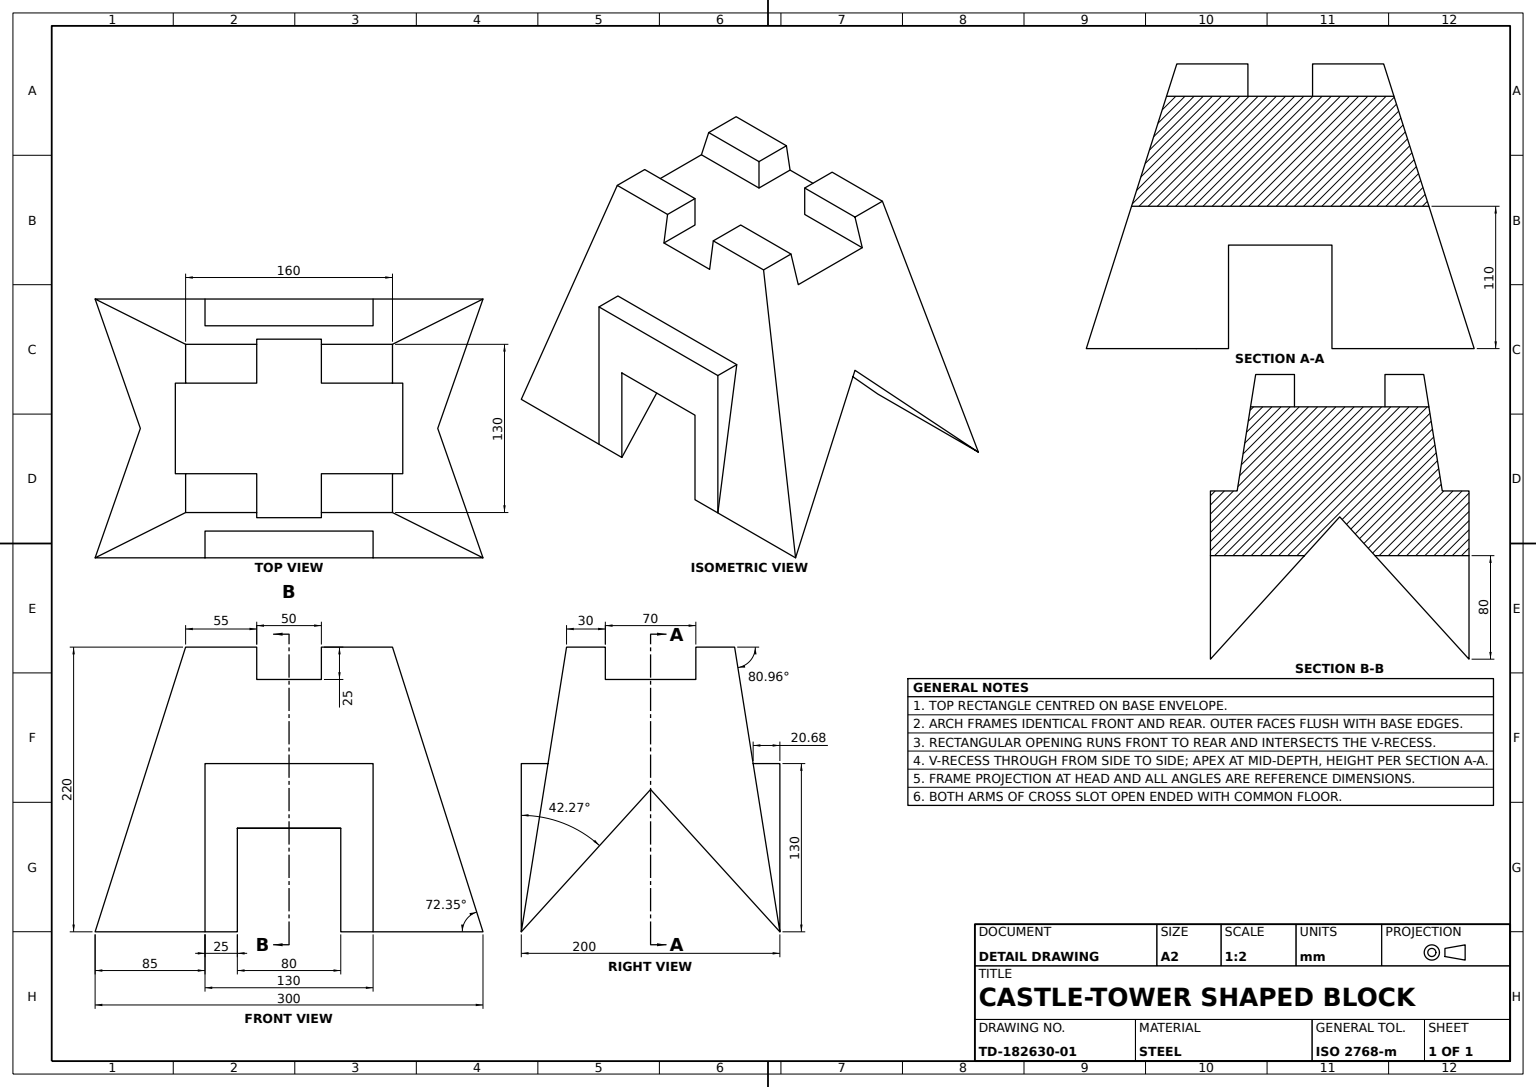
from build123d import *

# Parameters (mm, degrees)
INCLINED_BASE_BLOCK_DEPTH           = 100
FRONT_NOTCH_CUT_DEPTH               = 285.429253067
FRONT_NOTCH_CUT_DEPTH_BACK          = 285.429253067
FRONT_NOTCH_SKETCH_OUTSIDE_W        = 286.474
FRONT_NOTCH_SKETCH_OUTSIDE_H        = 306.474
TOP_RECESS_CUT_DEPTH                = 285.429253067
TOP_RECESS_CUT_DEPTH_BACK           = 285.429253067
FRONT_FRAME_BOSS_DEPTH              = 65
TOP_CROSS_SLOT_CUT_80X80_DEPTH      = 334.016516107
TOP_CROSS_SLOT_CUT_80X80_DEPTH_BACK = 334.016516107
TOP_CROSS_SLOT_SKETCH_W             = 80
TOP_CROSS_SLOT_SKETCH_H             = 80


with BuildPart() as part:
    # Base Profile Sketch → Inclined Base Block (new, symmetric)
    with BuildSketch(Plane(origin=(0, 0, 0), x_dir=(0, 0, -1), z_dir=(1, 0, 0))):
        Polygon((-150, 0), (-80, 220), (-25, 220), (-25, 195), (25, 195), (25, 220), (80, 220), (150, 0), align=None)
    extrude(amount=INCLINED_BASE_BLOCK_DEPTH, both=True)

    # Front Notch Sketch outside → Front Notch Cut (cut, two sides: drawn at the far end of the back side and taken through both)
    with BuildSketch(Plane.XY.offset(-FRONT_NOTCH_CUT_DEPTH_BACK)):
        with Locations((0, 110)):
            Rectangle(FRONT_NOTCH_SKETCH_OUTSIDE_W, FRONT_NOTCH_SKETCH_OUTSIDE_H)
        Polygon((-100, 0), (-65, 220), (-35, 220), (-35, 195), (35, 195), (35, 220), (65, 220), (100, 0), align=None, mode=Mode.SUBTRACT)
    extrude(amount=FRONT_NOTCH_CUT_DEPTH + FRONT_NOTCH_CUT_DEPTH_BACK, mode=Mode.SUBTRACT)

    # Top Recess Sketch → Top Recess Cut (cut, two sides: drawn at the far end of the back side and taken through both)
    with BuildSketch(Plane.XY.offset(-TOP_RECESS_CUT_DEPTH_BACK)):
        Polygon((-100, 0), (0, 110), (100, 0), align=None)
    extrude(amount=TOP_RECESS_CUT_DEPTH + TOP_RECESS_CUT_DEPTH_BACK, mode=Mode.SUBTRACT)

    # Front Frame Sketch → Front Frame Boss (add, symmetric)
    with BuildSketch(Plane.XY):
        Polygon((100, 0), (100, 130), (79.318181818, 130), align=None)
    front_frame_boss = extrude(amount=FRONT_FRAME_BOSS_DEPTH, both=True)

    # Front Frame Mirror: Front Frame Boss across plane
    add(front_frame_boss.mirror(Plane(origin=(0, 0, 0), x_dir=(0, 0, 1), z_dir=(1, 0, 0))))

    # Top Cross Slot Sketch → Top Cross Slot Cut 80x80 (cut, two sides: drawn at the far end of the back side and taken through both)
    with BuildSketch(Plane(origin=(100, 0, 0), x_dir=(0, 0, -1), z_dir=(1, 0, 0)).offset(-TOP_CROSS_SLOT_CUT_80X80_DEPTH_BACK)):
        with Locations((0, 40)):
            Rectangle(TOP_CROSS_SLOT_SKETCH_W, TOP_CROSS_SLOT_SKETCH_H)
    extrude(amount=TOP_CROSS_SLOT_CUT_80X80_DEPTH + TOP_CROSS_SLOT_CUT_80X80_DEPTH_BACK, mode=Mode.SUBTRACT)


solid = part.part
